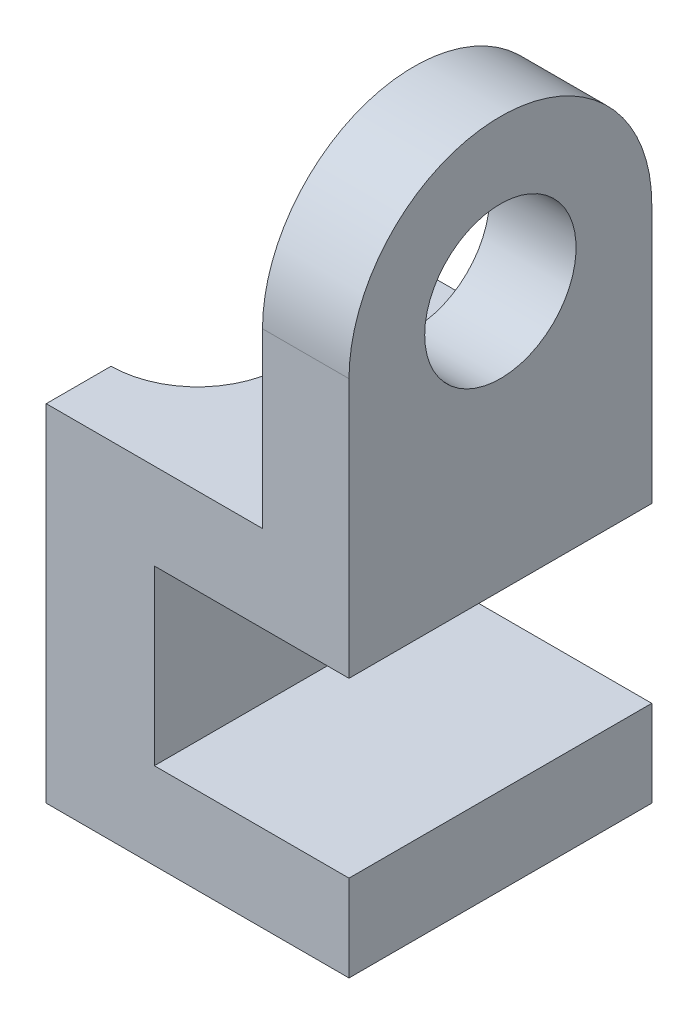
ISO-10303-21;
HEADER;
FILE_DESCRIPTION(('STEP AP214'),'2;1');
FILE_NAME('part.step','',(''),(''),'','','');
FILE_SCHEMA(('AUTOMOTIVE_DESIGN { 1 0 10303 214 1 1 1 1 }'));
ENDSEC;
DATA;
#1=APPLICATION_CONTEXT('core data for automotive mechanical design processes');
#2=APPLICATION_PROTOCOL_DEFINITION('international standard','automotive_design',2000,#1);
#3=PRODUCT_CONTEXT('',#1,'mechanical');
#4=PRODUCT('Part','Part','',(#3));
#5=PRODUCT_RELATED_PRODUCT_CATEGORY('part','',(#4));
#6=PRODUCT_DEFINITION_FORMATION('','',#4);
#7=PRODUCT_DEFINITION_CONTEXT('part definition',#1,'design');
#8=PRODUCT_DEFINITION('design','',#6,#7);
#9=PRODUCT_DEFINITION_SHAPE('','',#8);
#10=(LENGTH_UNIT() NAMED_UNIT(*) SI_UNIT(.MILLI.,.METRE.));
#11=(NAMED_UNIT(*) PLANE_ANGLE_UNIT() SI_UNIT($,.RADIAN.));
#12=(NAMED_UNIT(*) SI_UNIT($,.STERADIAN.) SOLID_ANGLE_UNIT());
#13=UNCERTAINTY_MEASURE_WITH_UNIT(LENGTH_MEASURE(1.E-05),#10,'distance_accuracy_value','');
#14=(GEOMETRIC_REPRESENTATION_CONTEXT(3) GLOBAL_UNCERTAINTY_ASSIGNED_CONTEXT((#13)) GLOBAL_UNIT_ASSIGNED_CONTEXT((#10,
#11,#12)) REPRESENTATION_CONTEXT('',''));
#15=CARTESIAN_POINT('',(0.,0.,0.));
#16=DIRECTION('',(0.,0.,1.));
#17=DIRECTION('',(1.,0.,0.));
#18=AXIS2_PLACEMENT_3D('',#15,#16,#17);
#19=CARTESIAN_POINT('',(0.,80.,70.));
#20=DIRECTION('',(1.,0.,0.));
#21=DIRECTION('',(0.,0.,-1.));
#22=AXIS2_PLACEMENT_3D('',#19,#20,#21);
#23=PLANE('',#22);
#24=DIRECTION('',(0.,0.,-1.));
#25=VECTOR('',#24,1.);
#26=CARTESIAN_POINT('',(0.,0.,70.));
#27=LINE('',#26,#25);
#28=CARTESIAN_POINT('',(0.,0.,15.));
#29=VERTEX_POINT('',#28);
#30=CARTESIAN_POINT('',(0.,0.,0.));
#31=VERTEX_POINT('',#30);
#32=EDGE_CURVE('E52',#29,#31,#27,.T.);
#33=ORIENTED_EDGE('',*,*,#32,.F.);
#34=DIRECTION('',(0.,1.,0.));
#35=VECTOR('',#34,1.);
#36=CARTESIAN_POINT('',(0.,0.,15.));
#37=LINE('',#36,#35);
#38=CARTESIAN_POINT('',(0.,80.,15.));
#39=VERTEX_POINT('',#38);
#40=EDGE_CURVE('E168',#29,#39,#37,.T.);
#41=ORIENTED_EDGE('',*,*,#40,.T.);
#42=DIRECTION('',(0.,0.,-1.));
#43=VECTOR('',#42,1.);
#44=CARTESIAN_POINT('',(0.,80.,70.));
#45=LINE('',#44,#43);
#46=CARTESIAN_POINT('',(0.,80.,0.));
#47=VERTEX_POINT('',#46);
#48=EDGE_CURVE('E192',#39,#47,#45,.T.);
#49=ORIENTED_EDGE('',*,*,#48,.T.);
#50=DIRECTION('',(0.,-1.,0.));
#51=VECTOR('',#50,1.);
#52=CARTESIAN_POINT('',(0.,80.,0.));
#53=LINE('',#52,#51);
#54=EDGE_CURVE('E174',#47,#31,#53,.T.);
#55=ORIENTED_EDGE('',*,*,#54,.T.);
#56=EDGE_LOOP('',(#33,#41,#49,#55));
#57=FACE_BOUND('',#56,.T.);
#58=ADVANCED_FACE('F44',(#57),#23,.F.);
#59=CARTESIAN_POINT('',(0.,80.,70.));
#60=VERTEX_POINT('',#59);
#61=CARTESIAN_POINT('',(0.,80.,55.));
#62=VERTEX_POINT('',#61);
#63=EDGE_CURVE('E208',#60,#62,#45,.T.);
#64=ORIENTED_EDGE('',*,*,#63,.T.);
#65=DIRECTION('',(0.,1.,0.));
#66=VECTOR('',#65,1.);
#67=CARTESIAN_POINT('',(0.,0.,55.));
#68=LINE('',#67,#66);
#69=CARTESIAN_POINT('',(0.,0.,55.));
#70=VERTEX_POINT('',#69);
#71=EDGE_CURVE('E69',#70,#62,#68,.T.);
#72=ORIENTED_EDGE('',*,*,#71,.F.);
#73=CARTESIAN_POINT('',(0.,0.,70.));
#74=VERTEX_POINT('',#73);
#75=EDGE_CURVE('E11',#74,#70,#27,.T.);
#76=ORIENTED_EDGE('',*,*,#75,.F.);
#77=DIRECTION('',(0.,-1.,0.));
#78=VECTOR('',#77,1.);
#79=CARTESIAN_POINT('',(0.,80.,70.));
#80=LINE('',#79,#78);
#81=EDGE_CURVE('E176',#60,#74,#80,.T.);
#82=ORIENTED_EDGE('',*,*,#81,.F.);
#83=EDGE_LOOP('',(#64,#72,#76,#82));
#84=FACE_BOUND('',#83,.T.);
#85=ADVANCED_FACE('F50',(#84),#23,.F.);
#86=CARTESIAN_POINT('',(0.,0.,70.));
#87=DIRECTION('',(0.,1.,0.));
#88=DIRECTION('',(0.,0.,1.));
#89=AXIS2_PLACEMENT_3D('',#86,#87,#88);
#90=PLANE('',#89);
#91=ORIENTED_EDGE('',*,*,#75,.T.);
#92=CARTESIAN_POINT('',(0.,0.,35.));
#93=DIRECTION('',(0.,1.,0.));
#94=DIRECTION('',(0.,0.,1.));
#95=AXIS2_PLACEMENT_3D('',#92,#93,#94);
#96=CIRCLE('',#95,20.);
#97=EDGE_CURVE('E170',#70,#29,#96,.T.);
#98=ORIENTED_EDGE('',*,*,#97,.T.);
#99=ORIENTED_EDGE('',*,*,#32,.T.);
#100=DIRECTION('',(1.,0.,0.));
#101=VECTOR('',#100,1.);
#102=CARTESIAN_POINT('',(0.,0.,0.));
#103=LINE('',#102,#101);
#104=CARTESIAN_POINT('',(70.,0.,0.));
#105=VERTEX_POINT('',#104);
#106=EDGE_CURVE('E195',#31,#105,#103,.T.);
#107=ORIENTED_EDGE('',*,*,#106,.T.);
#108=DIRECTION('',(0.,0.,-1.));
#109=VECTOR('',#108,1.);
#110=CARTESIAN_POINT('',(70.,0.,70.));
#111=LINE('',#110,#109);
#112=CARTESIAN_POINT('',(70.,0.,70.));
#113=VERTEX_POINT('',#112);
#114=EDGE_CURVE('E225',#113,#105,#111,.T.);
#115=ORIENTED_EDGE('',*,*,#114,.F.);
#116=DIRECTION('',(1.,0.,0.));
#117=VECTOR('',#116,1.);
#118=CARTESIAN_POINT('',(0.,0.,70.));
#119=LINE('',#118,#117);
#120=EDGE_CURVE('E179',#74,#113,#119,.T.);
#121=ORIENTED_EDGE('',*,*,#120,.F.);
#122=EDGE_LOOP('',(#91,#98,#99,#107,#115,#121));
#123=FACE_BOUND('',#122,.T.);
#124=ADVANCED_FACE('F231',(#123),#90,.F.);
#125=CARTESIAN_POINT('',(70.,0.,70.));
#126=DIRECTION('',(-1.,0.,0.));
#127=DIRECTION('',(0.,0.,1.));
#128=AXIS2_PLACEMENT_3D('',#125,#126,#127);
#129=PLANE('',#128);
#130=DIRECTION('',(0.,1.,0.));
#131=VECTOR('',#130,1.);
#132=CARTESIAN_POINT('',(70.,0.,0.));
#133=LINE('',#132,#131);
#134=CARTESIAN_POINT('',(70.,20.,0.));
#135=VERTEX_POINT('',#134);
#136=EDGE_CURVE('E197',#105,#135,#133,.T.);
#137=ORIENTED_EDGE('',*,*,#136,.T.);
#138=DIRECTION('',(0.,0.,-1.));
#139=VECTOR('',#138,1.);
#140=CARTESIAN_POINT('',(70.,20.,70.));
#141=LINE('',#140,#139);
#142=CARTESIAN_POINT('',(70.,20.,70.));
#143=VERTEX_POINT('',#142);
#144=EDGE_CURVE('E219',#143,#135,#141,.T.);
#145=ORIENTED_EDGE('',*,*,#144,.F.);
#146=DIRECTION('',(0.,1.,0.));
#147=VECTOR('',#146,1.);
#148=CARTESIAN_POINT('',(70.,0.,70.));
#149=LINE('',#148,#147);
#150=EDGE_CURVE('E182',#113,#143,#149,.T.);
#151=ORIENTED_EDGE('',*,*,#150,.F.);
#152=ORIENTED_EDGE('',*,*,#114,.T.);
#153=EDGE_LOOP('',(#137,#145,#151,#152));
#154=FACE_BOUND('',#153,.T.);
#155=ADVANCED_FACE('F261',(#154),#129,.F.);
#156=CARTESIAN_POINT('',(70.,20.,70.));
#157=DIRECTION('',(0.,-1.,0.));
#158=DIRECTION('',(0.,0.,-1.));
#159=AXIS2_PLACEMENT_3D('',#156,#157,#158);
#160=PLANE('',#159);
#161=DIRECTION('',(-1.,0.,0.));
#162=VECTOR('',#161,1.);
#163=CARTESIAN_POINT('',(70.,20.,0.));
#164=LINE('',#163,#162);
#165=CARTESIAN_POINT('',(25.,20.,0.));
#166=VERTEX_POINT('',#165);
#167=EDGE_CURVE('E200',#135,#166,#164,.T.);
#168=ORIENTED_EDGE('',*,*,#167,.T.);
#169=DIRECTION('',(0.,0.,-1.));
#170=VECTOR('',#169,1.);
#171=CARTESIAN_POINT('',(25.,20.,70.));
#172=LINE('',#171,#170);
#173=CARTESIAN_POINT('',(25.,20.,70.));
#174=VERTEX_POINT('',#173);
#175=EDGE_CURVE('E220',#174,#166,#172,.T.);
#176=ORIENTED_EDGE('',*,*,#175,.F.);
#177=DIRECTION('',(-1.,0.,0.));
#178=VECTOR('',#177,1.);
#179=CARTESIAN_POINT('',(70.,20.,70.));
#180=LINE('',#179,#178);
#181=EDGE_CURVE('E181',#143,#174,#180,.T.);
#182=ORIENTED_EDGE('',*,*,#181,.F.);
#183=ORIENTED_EDGE('',*,*,#144,.T.);
#184=EDGE_LOOP('',(#168,#176,#182,#183));
#185=FACE_BOUND('',#184,.T.);
#186=ADVANCED_FACE('F259',(#185),#160,.F.);
#187=CARTESIAN_POINT('',(25.,20.,70.));
#188=DIRECTION('',(-1.,0.,0.));
#189=DIRECTION('',(0.,0.,1.));
#190=AXIS2_PLACEMENT_3D('',#187,#188,#189);
#191=PLANE('',#190);
#192=DIRECTION('',(0.,1.,0.));
#193=VECTOR('',#192,1.);
#194=CARTESIAN_POINT('',(25.,20.,0.));
#195=LINE('',#194,#193);
#196=CARTESIAN_POINT('',(25.,60.,0.));
#197=VERTEX_POINT('',#196);
#198=EDGE_CURVE('E203',#166,#197,#195,.T.);
#199=ORIENTED_EDGE('',*,*,#198,.T.);
#200=DIRECTION('',(0.,0.,-1.));
#201=VECTOR('',#200,1.);
#202=CARTESIAN_POINT('',(25.,60.,70.));
#203=LINE('',#202,#201);
#204=CARTESIAN_POINT('',(25.,60.,70.));
#205=VERTEX_POINT('',#204);
#206=EDGE_CURVE('E212',#205,#197,#203,.T.);
#207=ORIENTED_EDGE('',*,*,#206,.F.);
#208=DIRECTION('',(0.,1.,0.));
#209=VECTOR('',#208,1.);
#210=CARTESIAN_POINT('',(25.,20.,70.));
#211=LINE('',#210,#209);
#212=EDGE_CURVE('E183',#174,#205,#211,.T.);
#213=ORIENTED_EDGE('',*,*,#212,.F.);
#214=ORIENTED_EDGE('',*,*,#175,.T.);
#215=EDGE_LOOP('',(#199,#207,#213,#214));
#216=FACE_BOUND('',#215,.T.);
#217=ADVANCED_FACE('F255',(#216),#191,.F.);
#218=CARTESIAN_POINT('',(25.,60.,70.));
#219=DIRECTION('',(0.,1.,0.));
#220=DIRECTION('',(0.,0.,1.));
#221=AXIS2_PLACEMENT_3D('',#218,#219,#220);
#222=PLANE('',#221);
#223=DIRECTION('',(1.,0.,0.));
#224=VECTOR('',#223,1.);
#225=CARTESIAN_POINT('',(25.,60.,0.));
#226=LINE('',#225,#224);
#227=CARTESIAN_POINT('',(70.,60.,0.));
#228=VERTEX_POINT('',#227);
#229=EDGE_CURVE('E201',#197,#228,#226,.T.);
#230=ORIENTED_EDGE('',*,*,#229,.T.);
#231=DIRECTION('',(0.,0.,-1.));
#232=VECTOR('',#231,1.);
#233=CARTESIAN_POINT('',(70.,60.,70.));
#234=LINE('',#233,#232);
#235=CARTESIAN_POINT('',(70.,60.,70.));
#236=VERTEX_POINT('',#235);
#237=EDGE_CURVE('E211',#236,#228,#234,.T.);
#238=ORIENTED_EDGE('',*,*,#237,.F.);
#239=DIRECTION('',(1.,0.,0.));
#240=VECTOR('',#239,1.);
#241=CARTESIAN_POINT('',(25.,60.,70.));
#242=LINE('',#241,#240);
#243=EDGE_CURVE('E187',#205,#236,#242,.T.);
#244=ORIENTED_EDGE('',*,*,#243,.F.);
#245=ORIENTED_EDGE('',*,*,#206,.T.);
#246=EDGE_LOOP('',(#230,#238,#244,#245));
#247=FACE_BOUND('',#246,.T.);
#248=ADVANCED_FACE('F250',(#247),#222,.F.);
#249=CARTESIAN_POINT('',(70.,60.,70.));
#250=DIRECTION('',(-1.,0.,0.));
#251=DIRECTION('',(0.,0.,1.));
#252=AXIS2_PLACEMENT_3D('',#249,#250,#251);
#253=PLANE('',#252);
#254=CARTESIAN_POINT('',(70.,120.,35.));
#255=DIRECTION('',(-1.,0.,0.));
#256=DIRECTION('',(0.,0.,1.));
#257=AXIS2_PLACEMENT_3D('',#254,#255,#256);
#258=CIRCLE('',#257,17.5);
#259=CARTESIAN_POINT('',(70.,120.,52.5));
#260=VERTEX_POINT('',#259);
#261=EDGE_CURVE('E160',#260,#260,#258,.T.);
#262=ORIENTED_EDGE('',*,*,#261,.T.);
#263=EDGE_LOOP('',(#262));
#264=FACE_BOUND('',#263,.T.);
#265=DIRECTION('',(0.,1.,0.));
#266=VECTOR('',#265,1.);
#267=CARTESIAN_POINT('',(70.,60.,0.));
#268=LINE('',#267,#266);
#269=CARTESIAN_POINT('',(70.,120.,0.));
#270=VERTEX_POINT('',#269);
#271=EDGE_CURVE('E202',#228,#270,#268,.T.);
#272=ORIENTED_EDGE('',*,*,#271,.T.);
#273=CARTESIAN_POINT('',(70.,120.,35.));
#274=DIRECTION('',(1.,0.,0.));
#275=DIRECTION('',(0.,0.,-1.));
#276=AXIS2_PLACEMENT_3D('',#273,#274,#275);
#277=CIRCLE('',#276,35.);
#278=CARTESIAN_POINT('',(70.,120.,70.));
#279=VERTEX_POINT('',#278);
#280=EDGE_CURVE('E154',#270,#279,#277,.T.);
#281=ORIENTED_EDGE('',*,*,#280,.T.);
#282=DIRECTION('',(0.,1.,0.));
#283=VECTOR('',#282,1.);
#284=CARTESIAN_POINT('',(70.,60.,70.));
#285=LINE('',#284,#283);
#286=EDGE_CURVE('E142',#236,#279,#285,.T.);
#287=ORIENTED_EDGE('',*,*,#286,.F.);
#288=ORIENTED_EDGE('',*,*,#237,.T.);
#289=EDGE_LOOP('',(#272,#281,#287,#288));
#290=FACE_BOUND('',#289,.T.);
#291=ADVANCED_FACE('F246',(#264,#290),#253,.F.);
#292=CARTESIAN_POINT('',(70.,80.,70.));
#293=DIRECTION('',(0.,-1.,0.));
#294=DIRECTION('',(0.,0.,-1.));
#295=AXIS2_PLACEMENT_3D('',#292,#293,#294);
#296=PLANE('',#295);
#297=DIRECTION('',(-1.,0.,0.));
#298=VECTOR('',#297,1.);
#299=CARTESIAN_POINT('',(70.,80.,70.));
#300=LINE('',#299,#298);
#301=CARTESIAN_POINT('',(50.,80.,70.));
#302=VERTEX_POINT('',#301);
#303=EDGE_CURVE('E190',#302,#60,#300,.T.);
#304=ORIENTED_EDGE('',*,*,#303,.F.);
#305=DIRECTION('',(0.,0.,-1.));
#306=VECTOR('',#305,1.);
#307=CARTESIAN_POINT('',(50.,80.,70.));
#308=LINE('',#307,#306);
#309=CARTESIAN_POINT('',(50.,80.,0.));
#310=VERTEX_POINT('',#309);
#311=EDGE_CURVE('E151',#302,#310,#308,.T.);
#312=ORIENTED_EDGE('',*,*,#311,.T.);
#313=DIRECTION('',(-1.,0.,0.));
#314=VECTOR('',#313,1.);
#315=CARTESIAN_POINT('',(70.,80.,0.));
#316=LINE('',#315,#314);
#317=EDGE_CURVE('E178',#310,#47,#316,.T.);
#318=ORIENTED_EDGE('',*,*,#317,.T.);
#319=ORIENTED_EDGE('',*,*,#48,.F.);
#320=CARTESIAN_POINT('',(0.,80.,35.));
#321=DIRECTION('',(0.,1.,0.));
#322=DIRECTION('',(0.,0.,1.));
#323=AXIS2_PLACEMENT_3D('',#320,#321,#322);
#324=CIRCLE('',#323,20.);
#325=EDGE_CURVE('E164',#62,#39,#324,.T.);
#326=ORIENTED_EDGE('',*,*,#325,.F.);
#327=ORIENTED_EDGE('',*,*,#63,.F.);
#328=EDGE_LOOP('',(#304,#312,#318,#319,#326,#327));
#329=FACE_BOUND('',#328,.T.);
#330=ADVANCED_FACE('F241',(#329),#296,.F.);
#331=CARTESIAN_POINT('',(0.,0.,70.));
#332=DIRECTION('',(0.,0.,1.));
#333=DIRECTION('',(1.,0.,0.));
#334=AXIS2_PLACEMENT_3D('',#331,#332,#333);
#335=PLANE('',#334);
#336=ORIENTED_EDGE('',*,*,#81,.T.);
#337=ORIENTED_EDGE('',*,*,#120,.T.);
#338=ORIENTED_EDGE('',*,*,#150,.T.);
#339=ORIENTED_EDGE('',*,*,#181,.T.);
#340=ORIENTED_EDGE('',*,*,#212,.T.);
#341=ORIENTED_EDGE('',*,*,#243,.T.);
#342=ORIENTED_EDGE('',*,*,#286,.T.);
#343=DIRECTION('',(1.,0.,0.));
#344=VECTOR('',#343,1.);
#345=CARTESIAN_POINT('',(50.,120.,70.));
#346=LINE('',#345,#344);
#347=CARTESIAN_POINT('',(50.,120.,70.));
#348=VERTEX_POINT('',#347);
#349=EDGE_CURVE('E135',#348,#279,#346,.T.);
#350=ORIENTED_EDGE('',*,*,#349,.F.);
#351=DIRECTION('',(0.,-1.,0.));
#352=VECTOR('',#351,1.);
#353=CARTESIAN_POINT('',(50.,120.,70.));
#354=LINE('',#353,#352);
#355=EDGE_CURVE('E138',#348,#302,#354,.T.);
#356=ORIENTED_EDGE('',*,*,#355,.T.);
#357=ORIENTED_EDGE('',*,*,#303,.T.);
#358=EDGE_LOOP('',(#336,#337,#338,#339,#340,#341,#342,#350,#356,#357));
#359=FACE_BOUND('',#358,.T.);
#360=ADVANCED_FACE('F139',(#359),#335,.T.);
#361=CARTESIAN_POINT('',(0.,0.,0.));
#362=DIRECTION('',(0.,0.,1.));
#363=DIRECTION('',(1.,0.,0.));
#364=AXIS2_PLACEMENT_3D('',#361,#362,#363);
#365=PLANE('',#364);
#366=ORIENTED_EDGE('',*,*,#54,.F.);
#367=ORIENTED_EDGE('',*,*,#317,.F.);
#368=DIRECTION('',(0.,1.,0.));
#369=VECTOR('',#368,1.);
#370=CARTESIAN_POINT('',(50.,80.,0.));
#371=LINE('',#370,#369);
#372=CARTESIAN_POINT('',(50.,120.,0.));
#373=VERTEX_POINT('',#372);
#374=EDGE_CURVE('E58',#310,#373,#371,.T.);
#375=ORIENTED_EDGE('',*,*,#374,.T.);
#376=DIRECTION('',(1.,0.,0.));
#377=VECTOR('',#376,1.);
#378=CARTESIAN_POINT('',(50.,120.,0.));
#379=LINE('',#378,#377);
#380=EDGE_CURVE('E150',#373,#270,#379,.T.);
#381=ORIENTED_EDGE('',*,*,#380,.T.);
#382=ORIENTED_EDGE('',*,*,#271,.F.);
#383=ORIENTED_EDGE('',*,*,#229,.F.);
#384=ORIENTED_EDGE('',*,*,#198,.F.);
#385=ORIENTED_EDGE('',*,*,#167,.F.);
#386=ORIENTED_EDGE('',*,*,#136,.F.);
#387=ORIENTED_EDGE('',*,*,#106,.F.);
#388=EDGE_LOOP('',(#366,#367,#375,#381,#382,#383,#384,#385,#386,#387));
#389=FACE_BOUND('',#388,.T.);
#390=ADVANCED_FACE('F235',(#389),#365,.F.);
#391=CARTESIAN_POINT('',(0.,0.,35.));
#392=DIRECTION('',(0.,1.,0.));
#393=DIRECTION('',(0.,0.,1.));
#394=AXIS2_PLACEMENT_3D('',#391,#392,#393);
#395=CYLINDRICAL_SURFACE('',#394,20.);
#396=ORIENTED_EDGE('',*,*,#325,.T.);
#397=ORIENTED_EDGE('',*,*,#40,.F.);
#398=ORIENTED_EDGE('',*,*,#97,.F.);
#399=ORIENTED_EDGE('',*,*,#71,.T.);
#400=EDGE_LOOP('',(#396,#397,#398,#399));
#401=FACE_BOUND('',#400,.T.);
#402=ADVANCED_FACE('F320',(#401),#395,.F.);
#403=CARTESIAN_POINT('',(50.,120.,35.));
#404=DIRECTION('',(1.,0.,0.));
#405=DIRECTION('',(0.,0.,-1.));
#406=AXIS2_PLACEMENT_3D('',#403,#404,#405);
#407=CYLINDRICAL_SURFACE('',#406,35.);
#408=ORIENTED_EDGE('',*,*,#280,.F.);
#409=ORIENTED_EDGE('',*,*,#380,.F.);
#410=CARTESIAN_POINT('',(50.,120.,35.));
#411=DIRECTION('',(1.,0.,0.));
#412=DIRECTION('',(0.,0.,-1.));
#413=AXIS2_PLACEMENT_3D('',#410,#411,#412);
#414=CIRCLE('',#413,35.);
#415=EDGE_CURVE('E147',#373,#348,#414,.T.);
#416=ORIENTED_EDGE('',*,*,#415,.T.);
#417=ORIENTED_EDGE('',*,*,#349,.T.);
#418=EDGE_LOOP('',(#408,#409,#416,#417));
#419=FACE_BOUND('',#418,.T.);
#420=ADVANCED_FACE('F153',(#419),#407,.T.);
#421=CARTESIAN_POINT('',(50.,120.,35.));
#422=DIRECTION('',(1.,0.,0.));
#423=DIRECTION('',(0.,0.,-1.));
#424=AXIS2_PLACEMENT_3D('',#421,#422,#423);
#425=PLANE('',#424);
#426=CARTESIAN_POINT('',(50.,120.,35.));
#427=DIRECTION('',(-1.,0.,0.));
#428=DIRECTION('',(0.,0.,1.));
#429=AXIS2_PLACEMENT_3D('',#426,#427,#428);
#430=CIRCLE('',#429,17.5);
#431=CARTESIAN_POINT('',(50.,120.,52.5));
#432=VERTEX_POINT('',#431);
#433=EDGE_CURVE('E159',#432,#432,#430,.T.);
#434=ORIENTED_EDGE('',*,*,#433,.F.);
#435=EDGE_LOOP('',(#434));
#436=FACE_BOUND('',#435,.T.);
#437=ORIENTED_EDGE('',*,*,#415,.F.);
#438=ORIENTED_EDGE('',*,*,#374,.F.);
#439=ORIENTED_EDGE('',*,*,#311,.F.);
#440=ORIENTED_EDGE('',*,*,#355,.F.);
#441=EDGE_LOOP('',(#437,#438,#439,#440));
#442=FACE_BOUND('',#441,.T.);
#443=ADVANCED_FACE('F149',(#436,#442),#425,.F.);
#444=CARTESIAN_POINT('',(70.,120.,35.));
#445=DIRECTION('',(-1.,0.,0.));
#446=DIRECTION('',(0.,0.,1.));
#447=AXIS2_PLACEMENT_3D('',#444,#445,#446);
#448=CYLINDRICAL_SURFACE('',#447,17.5);
#449=ORIENTED_EDGE('',*,*,#261,.F.);
#450=EDGE_LOOP('',(#449));
#451=FACE_BOUND('',#450,.T.);
#452=ORIENTED_EDGE('',*,*,#433,.T.);
#453=EDGE_LOOP('',(#452));
#454=FACE_BOUND('',#453,.T.);
#455=ADVANCED_FACE('F368',(#451,#454),#448,.F.);
#456=CLOSED_SHELL('',(#58,#85,#124,#155,#186,#217,#248,#291,#330,#360,#390,#402,#420,#443,#455));
#457=MANIFOLD_SOLID_BREP('B2',#456);
#458=ADVANCED_BREP_SHAPE_REPRESENTATION('',(#18,#457),#14);
#459=SHAPE_DEFINITION_REPRESENTATION(#9,#458);
ENDSEC;
END-ISO-10303-21;
